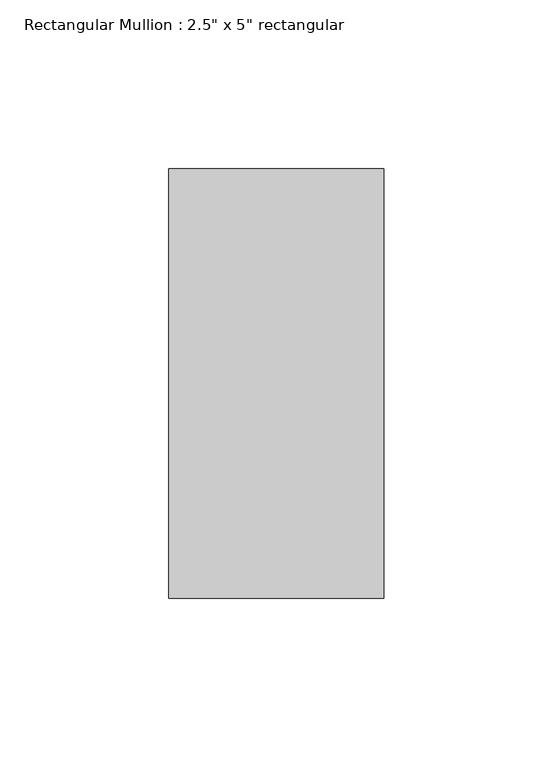
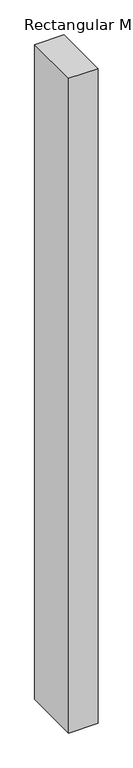
"""IFC4 building model written with IfcOpenShell, lengths in millimetres: member geometry."""

from ifc_helpers import new_model, si_unit, frame, origin, place, context, project, spatial, polyline, outline, extrude, source, transform, mapped, element, save


def member_c71c3647(model_context):
    return source(origin(), model_context, "Body", "SweptSolid", [
        extrude(outline(polyline([(31.75, 63.5), (31.75, -63.5), (-31.75, -63.5), (-31.75, 63.5), (31.75, 63.5)])), frame((0.0, 0.0, -1495.5694058), z_axis=(0.0, 0.0, 1.0), x_axis=(1.0, 0.0, 0.0)), (0.0, 0.0, 1.0), 1495.5694058),
    ])


if __name__ == "__main__":
    model = new_model("IFC4")
    model_context = context("Model", 3, world=origin())
    ifc_project = project(units=[si_unit("LENGTHUNIT", "METRE", prefix="MILLI")], contexts=[model_context])
    site = spatial("IfcSite", under=ifc_project)
    building = spatial("IfcBuilding", under=site)
    placement = place(None, origin())
    member_shape = member_c71c3647(model_context)
    element("IfcMember", 1, ObjectType="Rectangular Mullion : 2.5\" x 5\" rectangular", at=placement, inside=building, context=model_context, shape_type="MappedRepresentation", body=[
        mapped(member_shape, transform((0.0, 0.0, 0.0), x_axis=(1.0, 0.0, 0.0), y_axis=(0.0, 1.0, 0.0), z_axis=(0.0, 0.0, 1.0))),
    ])
    save(model, "model.ifc")

# Revit data of these elements
# Type "Rectangular Mullion : 2.5\" x 5\" rectangular"
#   built-in parameter 1007304 = 0.416667 (stored number, unit not read)
#   built-in parameter 1007301 = 0.104167 (stored number, unit not read)
#   built-in parameter 1007300 = 0.104167 (stored number, unit not read)
# Element 1 (IfcMember, "Rectangular Mullion : 2.5\" x 5\" rectangular")
#   Materials on its faces: "Aluminum"
# Materials
#   "Aluminum": class "Metal", colour RGB 247 247 247, transparency 0, Description = "Aluminum 6061", Cost = 0
